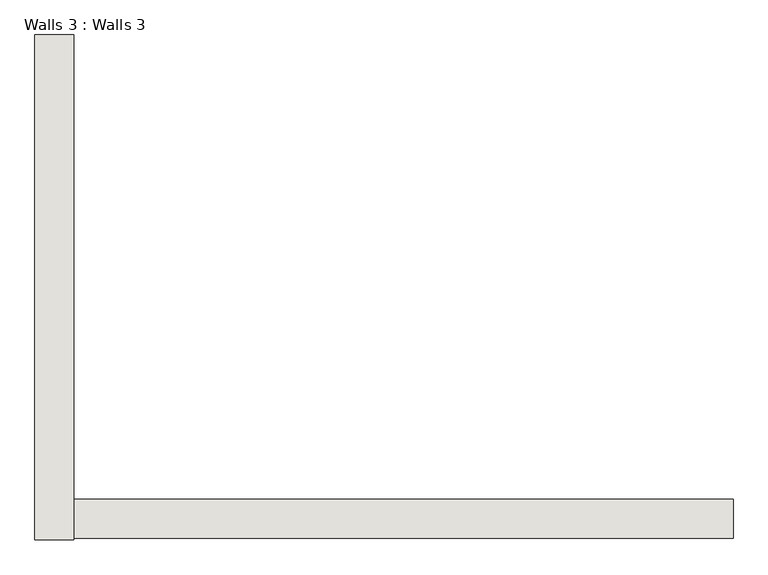
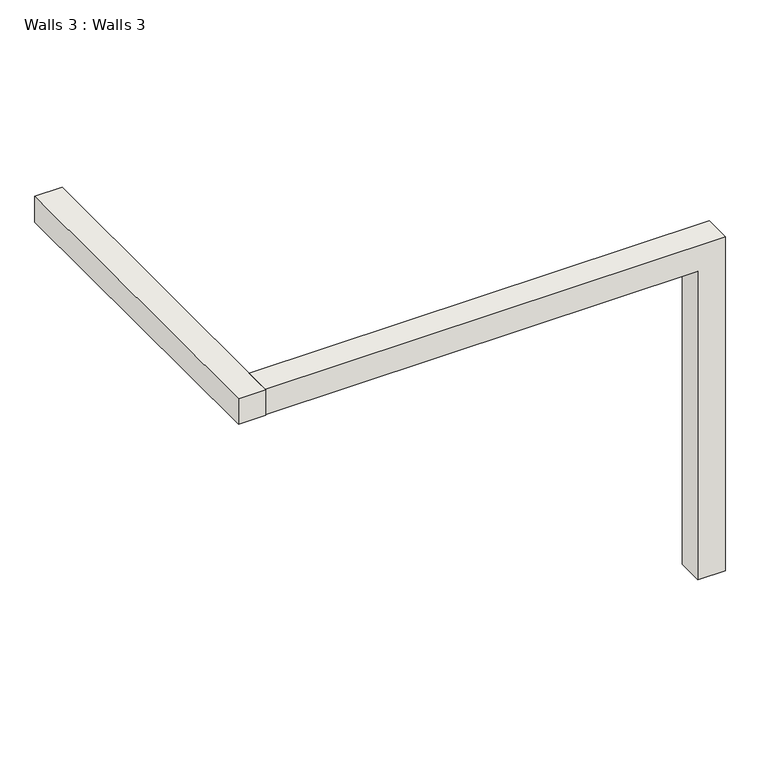
"""IFC4 building model written with IfcOpenShell, lengths in millimetres: wall geometry, Walls 3 : Walls 3."""

from ifc_helpers import new_model, si_unit, frame, origin, place, context, project, spatial, polyline, outline, extrude, source, transform, mapped, element, save


def walls_3_walls_3_b11343c7(model_context):
    return source(origin(), model_context, "Body", "SweptSolid", [
        extrude(outline(polyline([(-12000.149546, 5241.8756066), (-12000.149546, 9195.2170892), (-11695.349546, 9195.2170892), (-11695.349546, 5241.8756066), (-12000.149546, 5241.8756066)])), frame((0.0, 0.0, 7315.2), z_axis=(0.0, 0.0, 1.0), x_axis=(1.0, 0.0, 0.0)), (0.0, 0.0, 1.0), 304.8),
        extrude(outline(polyline([(7620.0, -11695.349546), (7315.2, -11695.349546), (7315.2, -6840.0943623), (3657.6, -6840.0943623), (3657.6, -6532.799546), (7620.0, -6532.799546), (7620.0, -11695.349546)])), frame((0.0, 5254.5756066, 0.0), z_axis=(0.0, 1.0, 0.0), x_axis=(0.0, 0.0, 1.0)), (0.0, 0.0, 1.0), 304.8),
    ])


if __name__ == "__main__":
    model = new_model("IFC4")
    model_context = context("Model", 3, world=origin())
    ifc_project = project(units=[si_unit("LENGTHUNIT", "METRE", prefix="MILLI")], contexts=[model_context])
    site = spatial("IfcSite", under=ifc_project)
    building = spatial("IfcBuilding", under=site)
    placement = place(None, origin())
    walls_3_walls_3_shape = walls_3_walls_3_b11343c7(model_context)
    element("IfcWall", 1, ObjectType="Walls 3 : Walls 3", at=placement, inside=building, context=model_context, shape_type="MappedRepresentation", body=[
        mapped(walls_3_walls_3_shape, transform((0.0, 0.0, 0.0), x_axis=(1.0, 0.0, 0.0), y_axis=(0.0, 1.0, 0.0), z_axis=(0.0, 0.0, 1.0))),
    ])
    save(model, "model.ifc")

# Revit data of these elements
# Element 1 (IfcWall, "Walls 3 : Walls 3")
#   Materials on its faces: "Default Wall"
# Materials
#   "Default Wall": colour RGB 128 128 128, transparency 0
